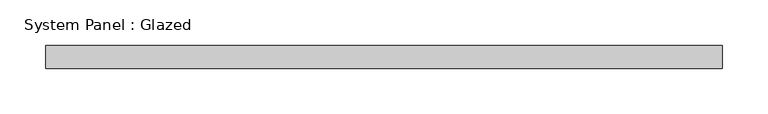
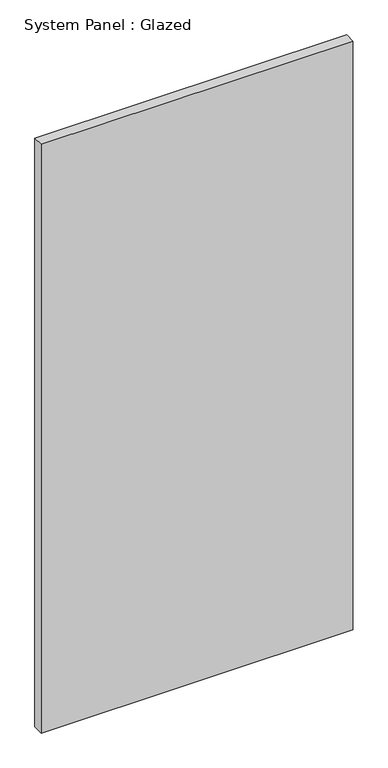
"""IFC4 building model written with IfcOpenShell, lengths in millimetres: plate geometry, System Panel : Glazed."""

from ifc_helpers import new_model, si_unit, origin, origin_with_axes, place, context, project, spatial, polyline, outline, extrude, source, transform, mapped, element, save


def system_panel_glazed_945fd4ba(model_context):
    return source(origin(), model_context, "Body", "SweptSolid", [
        extrude(outline(polyline([(371.475, 19.05), (-371.475, 19.05), (-371.475, 44.45), (371.475, 44.45), (371.475, 19.05)])), origin_with_axes(), (0.0, 0.0, 1.0), 1484.1494203),
    ])


if __name__ == "__main__":
    model = new_model("IFC4")
    model_context = context("Model", 3, world=origin())
    ifc_project = project(units=[si_unit("LENGTHUNIT", "METRE", prefix="MILLI")], contexts=[model_context])
    site = spatial("IfcSite", under=ifc_project)
    building = spatial("IfcBuilding", under=site)
    placement = place(None, origin())
    system_panel_glazed_shape = system_panel_glazed_945fd4ba(model_context)
    element("IfcPlate", 1, ObjectType="System Panel : Glazed", at=placement, inside=building, context=model_context, shape_type="MappedRepresentation", body=[
        mapped(system_panel_glazed_shape, transform((0.0, 0.0, 0.0), x_axis=(1.0, 0.0, 0.0), y_axis=(0.0, 1.0, 0.0), z_axis=(0.0, 0.0, 1.0))),
    ])
    save(model, "model.ifc")

# Revit data of these elements
# Type "System Panel : Glazed"
#   Construction Type Id = "GSP4R"
#   Analytic Construction = "1/8 in Pilkington single glazing"
#   Visual Light Transmittance = 0.9
#   Solar Heat Gain Coefficient = 0.86
#   Heat Transfer Coefficient (U) = 1.18115 BTU/(h·ft²·°F)
#   Define Thermal Properties by = 1
# Element 1 (IfcPlate, "System Panel : Glazed")
#   Materials on its faces: "Glass"
# Materials
#   "Glass": class "Glass", colour RGB 0 128 192, transparency 0.75, Description = "Soda Lime Glass", Cost = 0
